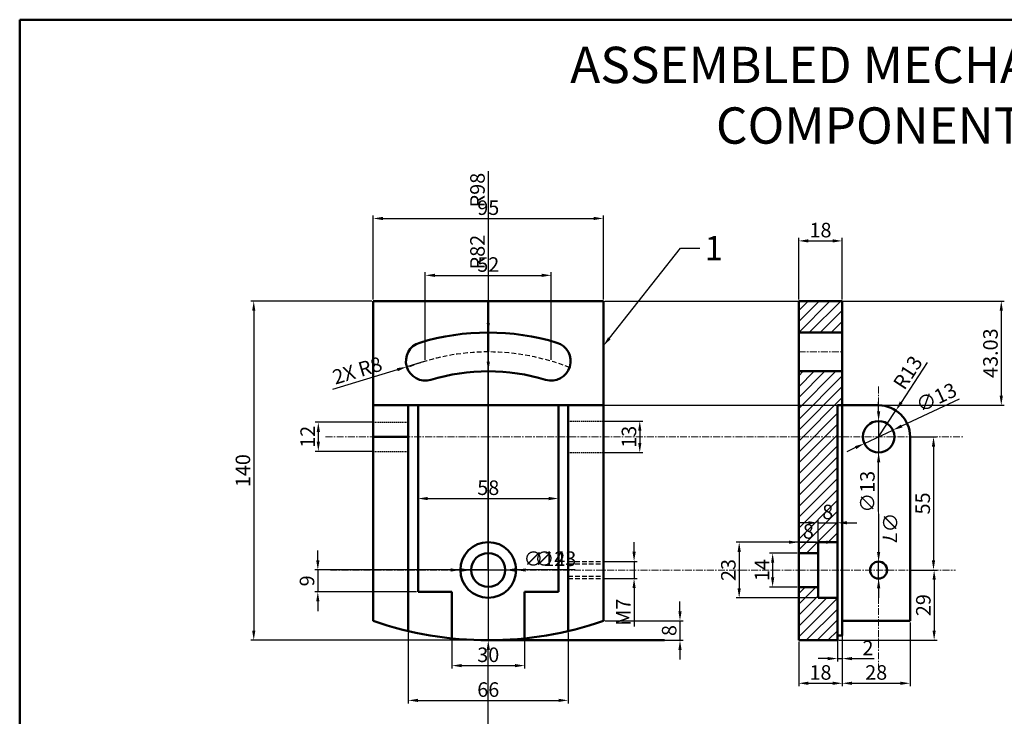
# Model space of a CAD drawing. Units: millimetres. Extents: x 197 to 841, y -182 to 351.
# Tile 2 of 3: x 197 to 603, y 63 to 351. Entities that reach past the tile are written whole.
import ezdxf
from ezdxf import colors
from ezdxf.entities.mleader import LeaderData, LeaderLine
from ezdxf.math import Vec2, Vec3

# ---------------------------------------------------------------- set-up
doc = ezdxf.new("R2010")
doc.units = ezdxf.units.MM
doc.header["$LTSCALE"] = 0.3
doc.linetypes.add('CENTER', pattern=[50.8, 31.75, -6.35, 6.35, -6.35])
doc.linetypes.add('HIDDEN', pattern=[9.525, 6.35, -3.175])
for name, color, linetype, lineweight in [('M-CNTR', 1, 'CENTER', 18), ('M-DIMS', 2, 'Continuous', 25), ('M-HATC', 8, 'Continuous', 18), ('M-HIDN', 6, 'HIDDEN', 25), ('M-OUTL', 7, 'Continuous', 50), ('M-TEXT', 3, 'Continuous', 25), ('M-TTLB', 7, 'Continuous', 50)]:
    doc.layers.add(name, color=color, linetype=linetype, lineweight=lineweight)
doc.styles.get("Standard").update_dxf_attribs({"font": 'arial.ttf'})
doc.dimstyles.new('ISO-25', dxfattribs={"dimtxt": 6, "dimasz": 4, "dimexe": 1.25, "dimexo": 0.625, "dimtad": 1, "dimdec": 0, "dimtxsty": 'Standard', "dimcen": 2.5, "dimadec": 0, "dimazin": 0, "dimtfac": 1, "dimtdec": 0, "dimtmove": 0, "dimatfit": 3, "dimfxl": 1, "dimarcsym": 0})

# ---------------------------------------------------------------- blocks, each defined once
blk = doc.blocks.new('*D1')
at = {"layer": 'Defpoints', "color": 0, "ltscale": 0.3, "transparency": 16777216}
for p in [(536.06, 98.08), (518.06, 94.62), (536.06, 76.86)]:
    blk.add_point(p, dxfattribs=at)
at = {"layer": 'M-DIMS', "color": 0, "lineweight": -2, "ltscale": 0.3, "transparency": 16777216}
for p, q in [((518.06, 94), (518.06, 75.61)), ((536.06, 97.46), (536.06, 75.61)), ((522.06, 76.86), (532.06, 76.86))]:
    blk.add_line(p, q, dxfattribs=at)
at = {"layer": 'M-DIMS', "color": 0, "ltscale": 0.3, "transparency": 16777216}
for points in [[(522.06, 77.52), (522.06, 76.19), (518.06, 76.86)], [(532.06, 77.52), (532.06, 76.19), (536.06, 76.86)]]:
    blk.add_solid(points, dxfattribs=at)
at = {"layer": 'M-DIMS', "color": 0, "ltscale": 0.3, "transparency": 16777216, "insert": (527.06, 80.55), "char_height": 6, "attachment_point": 5}
blk.add_mtext('18', dxfattribs=at)
blk = doc.blocks.new('*D2')
at = {"layer": 'Defpoints', "color": 0, "ltscale": 0.3, "transparency": 16777216}
for p in [(415.93, 245.24), (363.93, 209.78), (415.93, 209.78)]:
    blk.add_point(p, dxfattribs=at)
at = {"layer": 'M-DIMS', "color": 0, "lineweight": -2, "ltscale": 0.3, "transparency": 16777216}
for p, q in [((363.93, 210.41), (363.93, 246.49)), ((367.93, 245.24), (411.93, 245.24)), ((415.93, 210.41), (415.93, 246.49))]:
    blk.add_line(p, q, dxfattribs=at)
at = {"layer": 'M-DIMS', "color": 0, "ltscale": 0.3, "transparency": 16777216}
for points in [[(367.93, 245.91), (367.93, 244.58), (363.93, 245.24)], [(411.93, 245.91), (411.93, 244.58), (415.93, 245.24)]]:
    blk.add_solid(points, dxfattribs=at)
at = {"layer": 'M-DIMS', "color": 0, "ltscale": 0.3, "transparency": 16777216, "insert": (389.93, 248.93), "char_height": 6, "attachment_point": 5}
blk.add_mtext('52', dxfattribs=at)
blk = doc.blocks.new('*D3')
at = {"layer": 'Defpoints', "color": 0, "ltscale": 0.3, "transparency": 16777216}
for p in [(437.43, 268.71), (342.43, 234.62), (437.43, 234.62)]:
    blk.add_point(p, dxfattribs=at)
at = {"layer": 'M-DIMS', "color": 0, "lineweight": -2, "ltscale": 0.3, "transparency": 16777216}
for p, q in [((342.43, 235.25), (342.43, 269.96)), ((346.43, 268.71), (433.43, 268.71)), ((437.43, 235.25), (437.43, 269.96))]:
    blk.add_line(p, q, dxfattribs=at)
at = {"layer": 'M-DIMS', "color": 0, "ltscale": 0.3, "transparency": 16777216}
for points in [[(346.43, 269.38), (346.43, 268.05), (342.43, 268.71)], [(433.43, 269.38), (433.43, 268.05), (437.43, 268.71)]]:
    blk.add_solid(points, dxfattribs=at)
at = {"layer": 'M-DIMS', "color": 0, "ltscale": 0.3, "transparency": 16777216, "insert": (389.93, 272.4), "char_height": 6, "attachment_point": 5}
blk.add_mtext('95', dxfattribs=at)
blk = doc.blocks.new('*D4')
at = {"layer": 'Defpoints', "color": 0, "ltscale": 0.3, "transparency": 16777216}
for p in [(342.43, 234.62), (293.12, 94.62), (389.93, 94.62)]:
    blk.add_point(p, dxfattribs=at)
at = {"layer": 'M-DIMS', "color": 0, "lineweight": -2, "ltscale": 0.3, "transparency": 16777216}
for p, q in [((341.81, 234.62), (291.87, 234.62)), ((293.12, 230.62), (293.12, 98.62)), ((389.31, 94.62), (291.87, 94.62))]:
    blk.add_line(p, q, dxfattribs=at)
at = {"layer": 'M-DIMS', "color": 0, "ltscale": 0.3, "transparency": 16777216}
for points in [[(292.46, 230.62), (293.79, 230.62), (293.12, 234.62)], [(292.46, 98.62), (293.79, 98.62), (293.12, 94.62)]]:
    blk.add_solid(points, dxfattribs=at)
at = {"layer": 'M-DIMS', "color": 0, "ltscale": 0.3, "transparency": 16777216, "insert": (289.43, 164.62), "char_height": 6, "attachment_point": 5, "rotation": 90}
blk.add_mtext('140', dxfattribs=at)
blk = doc.blocks.new('*D5')
at = {"layer": 'Defpoints', "color": 0, "ltscale": 0.3, "transparency": 16777216}
for p in [(389.93, 123.62), (319.57, 114.62), (360.93, 114.62)]:
    blk.add_point(p, dxfattribs=at)
at = {"layer": 'M-DIMS', "color": 0, "lineweight": -2, "ltscale": 0.3, "transparency": 16777216}
for p, q in [((319.57, 127.62), (319.57, 131.62)), ((389.31, 123.62), (318.32, 123.62)), ((319.57, 123.62), (319.57, 114.62)), ((360.31, 114.62), (318.32, 114.62)), ((319.57, 110.62), (319.57, 106.62))]:
    blk.add_line(p, q, dxfattribs=at)
at = {"layer": 'M-DIMS', "color": 0, "ltscale": 0.3, "transparency": 16777216}
for points in [[(318.91, 127.62), (320.24, 127.62), (319.57, 123.62)], [(318.91, 110.62), (320.24, 110.62), (319.57, 114.62)]]:
    blk.add_solid(points, dxfattribs=at)
at = {"layer": 'M-DIMS', "color": 0, "ltscale": 0.3, "transparency": 16777216, "insert": (315.88, 119.12), "char_height": 6, "attachment_point": 5, "rotation": 90}
blk.add_mtext('9', dxfattribs=at)
blk = doc.blocks.new('*D6')
at = {"layer": 'Defpoints', "color": 0, "ltscale": 0.3, "transparency": 16777216}
for p in [(342.43, 184.59), (319.78, 172.59), (342.43, 172.59)]:
    blk.add_point(p, dxfattribs=at)
at = {"layer": 'M-DIMS', "color": 0, "lineweight": -2, "ltscale": 0.3, "transparency": 16777216}
for p, q in [((341.81, 184.59), (318.53, 184.59)), ((319.78, 180.59), (319.78, 176.59)), ((341.81, 172.59), (318.53, 172.59))]:
    blk.add_line(p, q, dxfattribs=at)
at = {"layer": 'M-DIMS', "color": 0, "ltscale": 0.3, "transparency": 16777216}
for points in [[(319.12, 180.59), (320.45, 180.59), (319.78, 184.59)], [(319.12, 176.59), (320.45, 176.59), (319.78, 172.59)]]:
    blk.add_solid(points, dxfattribs=at)
at = {"layer": 'M-DIMS', "color": 0, "ltscale": 0.3, "transparency": 16777216, "insert": (316.15, 178.59), "char_height": 6, "attachment_point": 5, "rotation": 90}
blk.add_mtext('12', dxfattribs=at)
blk = doc.blocks.new('*D7')
at = {"layer": 'Defpoints', "color": 0, "ltscale": 0.3, "transparency": 16777216}
for p in [(437.43, 185.09), (437.43, 172.09), (452.47, 172.09)]:
    blk.add_point(p, dxfattribs=at)
at = {"layer": 'M-DIMS', "color": 0, "lineweight": -2, "ltscale": 0.3, "transparency": 16777216}
for p, q in [((438.06, 185.09), (453.72, 185.09)), ((452.47, 181.09), (452.47, 176.09)), ((438.06, 172.09), (453.72, 172.09))]:
    blk.add_line(p, q, dxfattribs=at)
at = {"layer": 'M-DIMS', "color": 0, "ltscale": 0.3, "transparency": 16777216}
for points in [[(451.81, 181.09), (453.14, 181.09), (452.47, 185.09)], [(451.81, 176.09), (453.14, 176.09), (452.47, 172.09)]]:
    blk.add_solid(points, dxfattribs=at)
at = {"layer": 'M-DIMS', "color": 0, "ltscale": 0.3, "transparency": 16777216, "insert": (448.78, 178.59), "char_height": 6, "attachment_point": 5, "rotation": 90}
blk.add_mtext('13', dxfattribs=at)
blk = doc.blocks.new('*D8')
at = {"layer": 'Defpoints', "color": 0, "ltscale": 0.3, "transparency": 16777216}
for p in [(437.43, 127.12), (437.43, 120.12), (450.13, 120.12)]:
    blk.add_point(p, dxfattribs=at)
at = {"layer": 'M-DIMS', "color": 0, "lineweight": -2, "ltscale": 0.3, "transparency": 16777216}
for p, q in [((450.13, 131.12), (450.13, 135.12)), ((438.06, 127.12), (451.38, 127.12)), ((450.13, 127.12), (450.13, 120.12)), ((438.06, 120.12), (451.38, 120.12)), ((450.13, 116.12), (450.13, 100.23))]:
    blk.add_line(p, q, dxfattribs=at)
at = {"layer": 'M-DIMS', "color": 0, "ltscale": 0.3, "transparency": 16777216}
for points in [[(449.46, 131.12), (450.79, 131.12), (450.13, 127.12)], [(449.46, 116.12), (450.79, 116.12), (450.13, 120.12)]]:
    blk.add_solid(points, dxfattribs=at)
at = {"layer": 'M-DIMS', "color": 0, "ltscale": 0.3, "transparency": 16777216, "insert": (446.5, 106.18), "char_height": 6, "attachment_point": 5, "rotation": 90}
blk.add_mtext('M7', dxfattribs=at)
blk = doc.blocks.new('*D9')
at = {"layer": 'Defpoints', "color": 0, "ltscale": 0.3, "transparency": 16777216}
for p in [(360.93, 153.11), (418.93, 153.11), (418.93, 153.11)]:
    blk.add_point(p, dxfattribs=at)
at = {"layer": 'M-DIMS', "color": 0, "lineweight": -2, "ltscale": 0.3, "transparency": 16777216}
for p, q in [((360.93, 153.73), (360.93, 154.36)), ((364.93, 153.11), (414.93, 153.11)), ((418.93, 153.73), (418.93, 154.36))]:
    blk.add_line(p, q, dxfattribs=at)
at = {"layer": 'M-DIMS', "color": 0, "ltscale": 0.3, "transparency": 16777216}
for points in [[(364.93, 153.77), (364.93, 152.44), (360.93, 153.11)], [(414.93, 153.77), (414.93, 152.44), (418.93, 153.11)]]:
    blk.add_solid(points, dxfattribs=at)
at = {"layer": 'M-DIMS', "color": 0, "ltscale": 0.3, "transparency": 16777216, "insert": (389.93, 156.8), "char_height": 6, "attachment_point": 5}
blk.add_mtext('58', dxfattribs=at)
blk = doc.blocks.new('*D10')
at = {"layer": 'Defpoints', "color": 0, "ltscale": 0.3, "transparency": 16777216}
for p in [(374.93, 95.4), (404.93, 95.4), (404.93, 84.15)]:
    blk.add_point(p, dxfattribs=at)
at = {"layer": 'M-DIMS', "color": 0, "lineweight": -2, "ltscale": 0.3, "transparency": 16777216}
for p, q in [((374.93, 94.77), (374.93, 82.9)), ((404.93, 94.77), (404.93, 82.9)), ((378.93, 84.15), (400.93, 84.15))]:
    blk.add_line(p, q, dxfattribs=at)
at = {"layer": 'M-DIMS', "color": 0, "ltscale": 0.3, "transparency": 16777216}
for points in [[(378.93, 84.82), (378.93, 83.49), (374.93, 84.15)], [(400.93, 84.82), (400.93, 83.49), (404.93, 84.15)]]:
    blk.add_solid(points, dxfattribs=at)
at = {"layer": 'M-DIMS', "color": 0, "ltscale": 0.3, "transparency": 16777216, "insert": (389.93, 87.84), "char_height": 6, "attachment_point": 5}
blk.add_mtext('30', dxfattribs=at)
blk = doc.blocks.new('*D11')
at = {"layer": 'Defpoints', "color": 0, "ltscale": 0.3, "transparency": 16777216}
for p in [(356.93, 98.43), (422.93, 98.43), (422.93, 69.81)]:
    blk.add_point(p, dxfattribs=at)
at = {"layer": 'M-DIMS', "color": 0, "lineweight": -2, "ltscale": 0.3, "transparency": 16777216}
for p, q in [((356.93, 97.8), (356.93, 68.56)), ((422.93, 97.8), (422.93, 68.56)), ((360.93, 69.81), (418.93, 69.81))]:
    blk.add_line(p, q, dxfattribs=at)
at = {"layer": 'M-DIMS', "color": 0, "ltscale": 0.3, "transparency": 16777216}
for points in [[(360.93, 70.47), (360.93, 69.14), (356.93, 69.81)], [(418.93, 70.47), (418.93, 69.14), (422.93, 69.81)]]:
    blk.add_solid(points, dxfattribs=at)
at = {"layer": 'M-DIMS', "color": 0, "ltscale": 0.3, "transparency": 16777216, "insert": (389.93, 73.49), "char_height": 6, "attachment_point": 5}
blk.add_mtext('66', dxfattribs=at)
blk = doc.blocks.new('*D12')
at = {"layer": 'Defpoints', "color": 0, "ltscale": 0.3, "transparency": 16777216}
for p in [(437.43, 102.62), (437.43, 94.62), (469.07, 94.62)]:
    blk.add_point(p, dxfattribs=at)
at = {"layer": 'M-DIMS', "color": 0, "lineweight": -2, "ltscale": 0.3, "transparency": 16777216}
for p, q in [((469.07, 106.62), (469.07, 110.62)), ((438.06, 102.62), (470.32, 102.62)), ((469.07, 102.62), (469.07, 94.62)), ((438.06, 94.62), (470.32, 94.62)), ((469.07, 90.62), (469.07, 86.62))]:
    blk.add_line(p, q, dxfattribs=at)
at = {"layer": 'M-DIMS', "color": 0, "ltscale": 0.3, "transparency": 16777216}
for points in [[(468.41, 106.62), (469.74, 106.62), (469.07, 102.62)], [(468.41, 90.62), (469.74, 90.62), (469.07, 94.62)]]:
    blk.add_solid(points, dxfattribs=at)
at = {"layer": 'M-DIMS', "color": 0, "ltscale": 0.3, "transparency": 16777216, "insert": (465.38, 98.62), "char_height": 6, "attachment_point": 5, "rotation": 90}
blk.add_mtext('8', dxfattribs=at)
blk = doc.blocks.new('*D13')
at = {"layer": 'Defpoints', "color": 0, "ltscale": 0.3, "transparency": 16777216}
for p in [(536.06, 259.45), (518.06, 234.62), (536.06, 234.62)]:
    blk.add_point(p, dxfattribs=at)
at = {"layer": 'M-DIMS', "color": 0, "lineweight": -2, "ltscale": 0.3, "transparency": 16777216}
for p, q in [((518.06, 235.25), (518.06, 260.7)), ((536.06, 235.25), (536.06, 260.7)), ((522.06, 259.45), (532.06, 259.45))]:
    blk.add_line(p, q, dxfattribs=at)
at = {"layer": 'M-DIMS', "color": 0, "ltscale": 0.3, "transparency": 16777216}
for points in [[(522.06, 260.12), (522.06, 258.79), (518.06, 259.45)], [(532.06, 260.12), (532.06, 258.79), (536.06, 259.45)]]:
    blk.add_solid(points, dxfattribs=at)
at = {"layer": 'M-DIMS', "color": 0, "ltscale": 0.3, "transparency": 16777216, "insert": (527.06, 263.14), "char_height": 6, "attachment_point": 5}
blk.add_mtext('18', dxfattribs=at)
blk = doc.blocks.new('*D14')
at = {"layer": 'Defpoints', "color": 0, "ltscale": 0.3, "transparency": 16777216}
for p in [(564.06, 123.59), (534.06, 94.62), (573.98, 94.62)]:
    blk.add_point(p, dxfattribs=at)
at = {"layer": 'M-DIMS', "color": 0, "lineweight": -2, "ltscale": 0.3, "transparency": 16777216}
for p, q in [((564.69, 123.59), (575.23, 123.59)), ((573.98, 119.59), (573.98, 98.62)), ((534.69, 94.62), (575.23, 94.62))]:
    blk.add_line(p, q, dxfattribs=at)
at = {"layer": 'M-DIMS', "color": 0, "ltscale": 0.3, "transparency": 16777216}
for points in [[(573.32, 119.59), (574.65, 119.59), (573.98, 123.59)], [(573.32, 98.62), (574.65, 98.62), (573.98, 94.62)]]:
    blk.add_solid(points, dxfattribs=at)
at = {"layer": 'M-DIMS', "color": 0, "ltscale": 0.3, "transparency": 16777216, "insert": (570.3, 109.11), "char_height": 6, "attachment_point": 5, "rotation": 90}
blk.add_mtext('29', dxfattribs=at)
blk = doc.blocks.new('*D15')
at = {"layer": 'Defpoints', "color": 0, "ltscale": 0.3, "transparency": 16777216}
for p in [(564.06, 178.59), (564.06, 123.59), (573.72, 123.59)]:
    blk.add_point(p, dxfattribs=at)
at = {"layer": 'M-DIMS', "color": 0, "lineweight": -2, "ltscale": 0.3, "transparency": 16777216}
for p, q in [((564.69, 178.59), (574.97, 178.59)), ((573.72, 174.59), (573.72, 127.59)), ((564.69, 123.59), (574.97, 123.59))]:
    blk.add_line(p, q, dxfattribs=at)
at = {"layer": 'M-DIMS', "color": 0, "ltscale": 0.3, "transparency": 16777216}
for points in [[(573.05, 174.59), (574.38, 174.59), (573.72, 178.59)], [(573.05, 127.59), (574.38, 127.59), (573.72, 123.59)]]:
    blk.add_solid(points, dxfattribs=at)
at = {"layer": 'M-DIMS', "color": 0, "ltscale": 0.3, "transparency": 16777216, "insert": (570.04, 151.09), "char_height": 6, "attachment_point": 5, "rotation": 90}
blk.add_mtext('55', dxfattribs=at)
blk = doc.blocks.new('*D16')
at = {"layer": 'Defpoints', "color": 0, "ltscale": 0.3, "transparency": 16777216}
for p in [(518.06, 130.59), (507.31, 116.59), (518.06, 116.59)]:
    blk.add_point(p, dxfattribs=at)
at = {"layer": 'M-DIMS', "color": 0, "lineweight": -2, "ltscale": 0.3, "transparency": 16777216}
for p, q in [((517.44, 130.59), (506.06, 130.59)), ((507.31, 126.59), (507.31, 120.59)), ((517.44, 116.59), (506.06, 116.59))]:
    blk.add_line(p, q, dxfattribs=at)
at = {"layer": 'M-DIMS', "color": 0, "ltscale": 0.3, "transparency": 16777216}
for points in [[(506.64, 126.59), (507.98, 126.59), (507.31, 130.59)], [(506.64, 120.59), (507.98, 120.59), (507.31, 116.59)]]:
    blk.add_solid(points, dxfattribs=at)
at = {"layer": 'M-DIMS', "color": 0, "ltscale": 0.3, "transparency": 16777216, "insert": (503.67, 123.59), "char_height": 6, "attachment_point": 5, "rotation": 90}
blk.add_mtext('14', dxfattribs=at)
blk = doc.blocks.new('*D17')
at = {"layer": 'Defpoints', "color": 0, "ltscale": 0.3, "transparency": 16777216}
for p in [(526.06, 135.09), (493.5, 112.09), (526.06, 112.09)]:
    blk.add_point(p, dxfattribs=at)
at = {"layer": 'M-DIMS', "color": 0, "lineweight": -2, "ltscale": 0.3, "transparency": 16777216}
for p, q in [((525.44, 135.09), (492.25, 135.09)), ((493.5, 131.09), (493.5, 116.09)), ((525.44, 112.09), (492.25, 112.09))]:
    blk.add_line(p, q, dxfattribs=at)
at = {"layer": 'M-DIMS', "color": 0, "ltscale": 0.3, "transparency": 16777216}
for points in [[(492.83, 131.09), (494.17, 131.09), (493.5, 135.09)], [(492.83, 116.09), (494.17, 116.09), (493.5, 112.09)]]:
    blk.add_solid(points, dxfattribs=at)
at = {"layer": 'M-DIMS', "color": 0, "ltscale": 0.3, "transparency": 16777216, "insert": (489.81, 123.59), "char_height": 6, "attachment_point": 5, "rotation": 90}
blk.add_mtext('23', dxfattribs=at)
blk = doc.blocks.new('*D18')
at = {"layer": 'Defpoints', "color": 0, "ltscale": 0.3, "transparency": 16777216}
for p in [(564.06, 102.62), (536.06, 96.62), (564.06, 76.86)]:
    blk.add_point(p, dxfattribs=at)
at = {"layer": 'M-DIMS', "color": 0, "lineweight": -2, "ltscale": 0.3, "transparency": 16777216}
for p, q in [((564.06, 102), (564.06, 75.61)), ((536.06, 96), (536.06, 75.61)), ((540.06, 76.86), (560.06, 76.86))]:
    blk.add_line(p, q, dxfattribs=at)
at = {"layer": 'M-DIMS', "color": 0, "ltscale": 0.3, "transparency": 16777216}
for points in [[(540.06, 77.52), (540.06, 76.19), (536.06, 76.86)], [(560.06, 77.52), (560.06, 76.19), (564.06, 76.86)]]:
    blk.add_solid(points, dxfattribs=at)
at = {"layer": 'M-DIMS', "color": 0, "ltscale": 0.3, "transparency": 16777216, "insert": (550.06, 80.55), "char_height": 6, "attachment_point": 5}
blk.add_mtext('28', dxfattribs=at)
blk = doc.blocks.new('*D19')
at = {"layer": 'Defpoints', "color": 0, "ltscale": 0.3, "transparency": 16777216}
for p in [(534.06, 96.62), (536.06, 96.62), (536.06, 87.05)]:
    blk.add_point(p, dxfattribs=at)
at = {"layer": 'M-DIMS', "color": 0, "lineweight": -2, "ltscale": 0.3, "transparency": 16777216}
for p, q in [((534.06, 96), (534.06, 85.8)), ((536.06, 96), (536.06, 85.8)), ((530.06, 87.05), (526.06, 87.05)), ((534.06, 87.05), (536.06, 87.05)), ((540.06, 87.05), (549.28, 87.05))]:
    blk.add_line(p, q, dxfattribs=at)
at = {"layer": 'M-DIMS', "color": 0, "ltscale": 0.3, "transparency": 16777216}
for points in [[(530.06, 87.71), (530.06, 86.38), (534.06, 87.05)], [(540.06, 87.71), (540.06, 86.38), (536.06, 87.05)]]:
    blk.add_solid(points, dxfattribs=at)
at = {"layer": 'M-DIMS', "color": 0, "ltscale": 0.3, "transparency": 16777216, "insert": (546.67, 90.68), "char_height": 6, "attachment_point": 5}
blk.add_mtext('2', dxfattribs=at)
blk = doc.blocks.new('*D20')
at = {"layer": 'Defpoints', "color": 0, "ltscale": 0.3, "transparency": 16777216}
for p in [(534.06, 143.11), (526.06, 135.09), (534.06, 135.09)]:
    blk.add_point(p, dxfattribs=at)
at = {"layer": 'M-DIMS', "color": 0, "lineweight": -2, "ltscale": 0.3, "transparency": 16777216}
for p, q in [((522.06, 143.11), (518.06, 143.11)), ((526.06, 135.72), (526.06, 144.36)), ((526.06, 143.11), (534.06, 143.11)), ((534.06, 135.72), (534.06, 144.36)), ((538.06, 143.11), (542.06, 143.11))]:
    blk.add_line(p, q, dxfattribs=at)
at = {"layer": 'M-DIMS', "color": 0, "ltscale": 0.3, "transparency": 16777216}
for points in [[(522.06, 143.77), (522.06, 142.44), (526.06, 143.11)], [(538.06, 143.77), (538.06, 142.44), (534.06, 143.11)]]:
    blk.add_solid(points, dxfattribs=at)
at = {"layer": 'M-DIMS', "color": 0, "ltscale": 0.3, "transparency": 16777216, "insert": (530.06, 146.8), "char_height": 6, "attachment_point": 5}
blk.add_mtext('8', dxfattribs=at)
blk = doc.blocks.new('*D21')
at = {"layer": 'Defpoints', "color": 0, "ltscale": 0.3, "transparency": 16777216}
for p in [(526.06, 135.09), (518.06, 130.59), (526.06, 130.59)]:
    blk.add_point(p, dxfattribs=at)
at = {"layer": 'M-DIMS', "color": 0, "lineweight": -2, "ltscale": 0.3, "transparency": 16777216}
for p, q in [((514.06, 135.09), (510.06, 135.09)), ((518.06, 131.22), (518.06, 136.34)), ((518.06, 135.09), (526.06, 135.09)), ((526.06, 131.22), (526.06, 136.34)), ((530.06, 135.09), (534.06, 135.09))]:
    blk.add_line(p, q, dxfattribs=at)
at = {"layer": 'M-DIMS', "color": 0, "ltscale": 0.3, "transparency": 16777216}
for points in [[(514.06, 135.76), (514.06, 134.43), (518.06, 135.09)], [(530.06, 135.76), (530.06, 134.43), (526.06, 135.09)]]:
    blk.add_solid(points, dxfattribs=at)
at = {"layer": 'M-DIMS', "color": 0, "ltscale": 0.3, "transparency": 16777216, "insert": (522.06, 138.78), "char_height": 6, "attachment_point": 5}
blk.add_mtext('8', dxfattribs=at)
blk = doc.blocks.new('*D22')
at = {"layer": 'Defpoints', "color": 0, "ltscale": 0.3, "transparency": 16777216}
for p in [(558.18, 189.47), (551.06, 178.59)]:
    blk.add_point(p, dxfattribs=at)
at = {"layer": 'M-DIMS', "color": 0, "lineweight": -2, "ltscale": 0.3, "transparency": 16777216}
for p, q in [((571.11, 209.2), (560.38, 192.81)), ((551.06, 178.59), (558.18, 189.47))]:
    blk.add_line(p, q, dxfattribs=at)
at = {"layer": 'M-DIMS', "color": 0, "ltscale": 0.3, "transparency": 16777216}
blk.add_solid([(559.82, 193.18), (560.93, 192.45), (558.18, 189.47)], dxfattribs=at)
at = {"layer": 'M-DIMS', "color": 0, "ltscale": 0.3, "transparency": 16777216, "insert": (563.75, 204.7), "char_height": 6, "attachment_point": 5, "rotation": 56.7737}
blk.add_mtext('R13', dxfattribs=at)
blk = doc.blocks.new('*D23')
at = {"layer": 'Defpoints', "color": 0, "ltscale": 0.3, "transparency": 16777216}
for p in [(556.95, 181.35), (545.17, 175.84)]:
    blk.add_point(p, dxfattribs=at)
at = {"layer": 'M-DIMS', "color": 0, "lineweight": -2, "ltscale": 0.3, "transparency": 16777216}
for p, q in [((584.27, 194.14), (560.57, 183.05)), ((545.17, 175.84), (556.95, 181.35)), ((541.55, 174.14), (537.93, 172.44))]:
    blk.add_line(p, q, dxfattribs=at)
at = {"layer": 'M-DIMS', "color": 0, "ltscale": 0.3, "transparency": 16777216}
for points in [[(560.29, 183.65), (560.85, 182.44), (556.95, 181.35)], [(541.27, 174.74), (541.83, 173.54), (545.17, 175.84)]]:
    blk.add_solid(points, dxfattribs=at)
at = {"layer": 'M-DIMS', "color": 0, "ltscale": 0.3, "transparency": 16777216, "insert": (575.22, 194.16), "char_height": 6, "attachment_point": 5, "rotation": 25.0912}
blk.add_mtext('∅13', dxfattribs=at)
blk = doc.blocks.new('*D64')
at = {"layer": 'Defpoints', "color": 0, "ltscale": 0.3, "transparency": 16777216}
for p in [(437.43, 234.62), (437.43, 191.59), (601.69, 191.59)]:
    blk.add_point(p, dxfattribs=at)
at = {"layer": 'M-DIMS', "color": 0, "lineweight": -2, "ltscale": 0.3, "transparency": 16777216}
for p, q in [((438.06, 234.62), (602.94, 234.62)), ((601.69, 230.62), (601.69, 195.59)), ((438.06, 191.59), (602.94, 191.59))]:
    blk.add_line(p, q, dxfattribs=at)
at = {"layer": 'M-DIMS', "color": 0, "ltscale": 0.3, "transparency": 16777216}
for points in [[(601.02, 230.62), (602.36, 230.62), (601.69, 234.62)], [(601.02, 195.59), (602.36, 195.59), (601.69, 191.59)]]:
    blk.add_solid(points, dxfattribs=at)
at = {"layer": 'M-DIMS', "color": 0, "ltscale": 0.3, "transparency": 16777216, "insert": (598, 213.11), "char_height": 6, "attachment_point": 5, "rotation": 90}
blk.add_mtext('43.03', dxfattribs=at)
blk = doc.blocks.new('*D67')
at = {"layer": 'Defpoints', "color": 0, "ltscale": 0.3, "transparency": 16777216}
for p in [(356.28, 207.47), (363.93, 209.78)]:
    blk.add_point(p, dxfattribs=at)
at = {"layer": 'M-DIMS', "color": 0, "lineweight": -2, "ltscale": 0.3, "transparency": 16777216}
for p, q in [((363.93, 209.78), (356.28, 207.47)), ((325.71, 198.25), (352.45, 206.32))]:
    blk.add_line(p, q, dxfattribs=at)
at = {"layer": 'M-DIMS', "color": 0, "ltscale": 0.3, "transparency": 16777216}
blk.add_solid([(352.25, 206.95), (352.64, 205.68), (356.28, 207.47)], dxfattribs=at)
at = {"layer": 'M-DIMS', "color": 0, "ltscale": 0.3, "transparency": 16777216, "insert": (336.1, 205.23), "char_height": 6, "attachment_point": 5, "rotation": 16.7934}
blk.add_mtext('2X R8', dxfattribs=at)
blk = doc.blocks.new('*D68')
at = {"layer": 'Defpoints', "color": 0, "ltscale": 0.3, "transparency": 16777216}
for p in [(389.94, 221.62), (389.93, 123.62)]:
    blk.add_point(p, dxfattribs=at)
at = {"layer": 'M-DIMS', "color": 0, "lineweight": -2, "ltscale": 0.3, "transparency": 16777216}
for p, q in [((389.94, 288.22), (389.94, 225.62)), ((389.93, 123.62), (389.94, 221.62))]:
    blk.add_line(p, q, dxfattribs=at)
at = {"layer": 'M-DIMS', "color": 0, "ltscale": 0.3, "transparency": 16777216}
blk.add_solid([(389.27, 225.62), (390.6, 225.62), (389.94, 221.62)], dxfattribs=at)
at = {"layer": 'M-DIMS', "color": 0, "ltscale": 0.3, "transparency": 16777216, "insert": (386.25, 280.42), "char_height": 6, "attachment_point": 5, "rotation": 89.9999}
blk.add_mtext('R98', dxfattribs=at)
blk = doc.blocks.new('*D69')
at = {"layer": 'Defpoints', "color": 0, "ltscale": 0.3, "transparency": 16777216}
for p in [(389.93, 205.62), (389.93, 123.62)]:
    blk.add_point(p, dxfattribs=at)
at = {"layer": 'M-DIMS', "color": 0, "lineweight": -2, "ltscale": 0.3, "transparency": 16777216}
for p, q in [((389.94, 262.58), (389.93, 209.62)), ((389.93, 123.62), (389.93, 205.62))]:
    blk.add_line(p, q, dxfattribs=at)
at = {"layer": 'M-DIMS', "color": 0, "ltscale": 0.3, "transparency": 16777216}
blk.add_solid([(389.27, 209.62), (390.6, 209.62), (389.93, 205.62)], dxfattribs=at)
at = {"layer": 'M-DIMS', "color": 0, "ltscale": 0.3, "transparency": 16777216, "insert": (386.25, 254.82), "char_height": 6, "attachment_point": 5, "rotation": 89.9999}
blk.add_mtext('R82', dxfattribs=at)
blk = doc.blocks.new('*D70')
at = {"layer": 'Defpoints', "color": 0, "ltscale": 0.3, "transparency": 16777216}
for p in [(389.93, 239.64), (389.94, 94.62)]:
    blk.add_point(p, dxfattribs=at)
at = {"layer": 'M-DIMS', "color": 0, "lineweight": -2, "ltscale": 0.3, "transparency": 16777216}
for p, q in [((389.93, 239.64), (389.94, 94.62)), ((389.94, -8.31), (389.94, 90.62))]:
    blk.add_line(p, q, dxfattribs=at)
at = {"layer": 'M-DIMS', "color": 0, "ltscale": 0.3, "transparency": 16777216}
blk.add_solid([(390.6, 90.62), (389.27, 90.62), (389.94, 94.62)], dxfattribs=at)
at = {"layer": 'M-DIMS', "color": 0, "ltscale": 0.3, "transparency": 16777216, "insert": (393.62, 7.61), "char_height": 6, "attachment_point": 5, "rotation": 270.0001}
blk.add_mtext('R145.02', dxfattribs=at)
blk = doc.blocks.new('*D71')
at = {"layer": 'Defpoints', "color": 0, "ltscale": 0.3, "transparency": 16777216}
for p in [(378.43, 123.62), (401.43, 123.62)]:
    blk.add_point(p, dxfattribs=at)
at = {"layer": 'M-DIMS', "color": 0, "lineweight": -2, "ltscale": 0.3, "transparency": 16777216}
for p, q in [((374.43, 123.62), (370.43, 123.62)), ((378.43, 123.62), (401.43, 123.62)), ((425.81, 123.62), (405.43, 123.62))]:
    blk.add_line(p, q, dxfattribs=at)
at = {"layer": 'M-DIMS', "color": 0, "ltscale": 0.3, "transparency": 16777216}
for points in [[(374.43, 124.29), (374.43, 122.95), (378.43, 123.62)], [(405.43, 124.29), (405.43, 122.95), (401.43, 123.62)]]:
    blk.add_solid(points, dxfattribs=at)
at = {"layer": 'M-DIMS', "color": 0, "ltscale": 0.3, "transparency": 16777216, "insert": (417.62, 127.48), "char_height": 6, "attachment_point": 5, "rotation": 0.0013}
blk.add_mtext('∅23', dxfattribs=at)
blk = doc.blocks.new('*D72')
at = {"layer": 'Defpoints', "color": 0, "ltscale": 0.3, "transparency": 16777216}
for p in [(382.93, 123.62), (396.93, 123.62)]:
    blk.add_point(p, dxfattribs=at)
at = {"layer": 'M-DIMS', "color": 0, "lineweight": -2, "ltscale": 0.3, "transparency": 16777216}
for p, q in [((378.93, 123.62), (374.93, 123.62)), ((382.93, 123.62), (396.93, 123.62)), ((421.28, 123.62), (400.93, 123.62))]:
    blk.add_line(p, q, dxfattribs=at)
at = {"layer": 'M-DIMS', "color": 0, "ltscale": 0.3, "transparency": 16777216}
for points in [[(378.93, 124.29), (378.93, 122.95), (382.93, 123.62)], [(400.93, 124.29), (400.93, 122.95), (396.93, 123.62)]]:
    blk.add_solid(points, dxfattribs=at)
at = {"layer": 'M-DIMS', "color": 0, "ltscale": 0.3, "transparency": 16777216, "insert": (413.11, 127.48), "char_height": 6, "attachment_point": 5, "rotation": 0.0022}
blk.add_mtext('∅14', dxfattribs=at)
blk = doc.blocks.new('*D73')
at = {"layer": 'Defpoints', "color": 0, "ltscale": 0.3, "transparency": 16777216}
for p in [(551.06, 185.09), (551.06, 172.09)]:
    blk.add_point(p, dxfattribs=at)
at = {"layer": 'M-DIMS', "color": 0, "lineweight": -2, "ltscale": 0.3, "transparency": 16777216}
for p, q in [((551.06, 189.09), (551.06, 193.09)), ((551.06, 185.09), (551.06, 172.09)), ((551.06, 147.72), (551.06, 168.09))]:
    blk.add_line(p, q, dxfattribs=at)
at = {"layer": 'M-DIMS', "color": 0, "ltscale": 0.3, "transparency": 16777216}
for points in [[(550.39, 189.09), (551.73, 189.09), (551.06, 185.09)], [(550.39, 168.09), (551.73, 168.09), (551.06, 172.09)]]:
    blk.add_solid(points, dxfattribs=at)
at = {"layer": 'M-DIMS', "color": 0, "ltscale": 0.3, "transparency": 16777216, "insert": (547.2, 155.91), "char_height": 6, "attachment_point": 5, "rotation": 89.9987}
blk.add_mtext('∅13', dxfattribs=at)
blk = doc.blocks.new('*D74')
at = {"layer": 'Defpoints', "color": 0, "ltscale": 0.3, "transparency": 16777216}
for p in [(551.06, 127.09), (551.06, 120.09)]:
    blk.add_point(p, dxfattribs=at)
at = {"layer": 'M-DIMS', "color": 0, "lineweight": -2, "ltscale": 0.3, "transparency": 16777216}
for p, q in [((551.06, 146.8), (551.06, 131.09)), ((551.06, 120.09), (551.06, 127.09)), ((551.06, 116.09), (551.06, 112.09))]:
    blk.add_line(p, q, dxfattribs=at)
at = {"layer": 'M-DIMS', "color": 0, "ltscale": 0.3, "transparency": 16777216}
for points in [[(551.73, 131.09), (550.39, 131.09), (551.06, 127.09)], [(551.73, 116.09), (550.39, 116.09), (551.06, 120.09)]]:
    blk.add_solid(points, dxfattribs=at)
at = {"layer": 'M-DIMS', "color": 0, "ltscale": 0.3, "transparency": 16777216, "insert": (554.92, 140.95), "char_height": 6, "attachment_point": 5, "rotation": 270.0025}
blk.add_mtext('∅7', dxfattribs=at)

msp = doc.modelspace()

# ---------------------------------------------------------------- hatches: boundary and pattern name
at = {"layer": 'M-HATC', "ltscale": 0.3}
h = msp.add_hatch(dxfattribs=at)
h.set_pattern_fill('ANSI31', color=256)
h.paths.add_polyline_path([(534.0602, 178.5927), (518.0602, 178.5927), (518.0602, 130.5927), (526.0602, 130.5927), (526.0602, 135.0927), (534.0602, 135.0927)])
h.paths.add_polyline_path([(534.0602, 112.0927), (526.0602, 112.0927), (526.0602, 116.5927), (518.0602, 116.5927), (518.0602, 94.6207), (534.0602, 94.6207)])
h.paths.add_polyline_path([(536.0602, 205.6207), (518.0602, 205.6207), (518.0602, 178.5927), (534.0602, 178.5927), (534.0602, 191.5927), (536.0602, 191.5927)])
h.paths.add_polyline_path([(536.0602, 234.6207), (518.0602, 234.6207), (518.0602, 221.6207), (536.0602, 221.6207)])

# ---------------------------------------------------------------- linework, layer by layer
at = {"layer": 'M-CNTR'}
msp.add_line((389.9348, 234.6207), (389.9348, 94.6207), dxfattribs=at)
at = {"layer": 'M-CNTR', "ltscale": 0.3}
for p, q in [((518.0602, 213.6207), (536.0602, 213.6207)), ((551.0602, 199.3431), (551.0602, 83.5004)), ((322.7995, 178.5927), (536.0602, 178.5927)), ((536.0602, 178.5927), (586.0907, 178.5927)), ((324.7426, 123.5927), (518.0602, 123.5927)), ((518.0602, 123.5927), (582.811, 123.5927))]:
    msp.add_line(p, q, dxfattribs=at)
at = {"layer": 'M-HIDN', "ltscale": 0.3}
for p, q in [((342.4348, 184.5927), (356.9348, 184.5927)), ((422.9348, 185.0927), (437.4348, 185.0927)), ((342.4348, 172.5927), (356.9348, 172.5927)), ((422.9348, 172.0927), (437.4348, 172.0927))]:
    msp.add_line(p, q, dxfattribs=at)
at = {"layer": 'M-HIDN'}
for p, q in [((422.9348, 127.1207), (437.4348, 127.1207)), ((422.9348, 126.1207), (437.4348, 126.1207)), ((422.9348, 121.1207), (437.4348, 121.1207)), ((422.9348, 120.1207), (437.4348, 120.1207))]:
    msp.add_line(p, q, dxfattribs=at)
msp.add_arc((389.9348, 123.6207), 90, 68.113917, 111.886083, dxfattribs=at)
at = {"layer": 'M-OUTL'}
for p, q in [((342.4348, 234.6207), (437.4348, 234.6207)), ((342.4348, 102.6207), (342.4348, 234.6207)), ((389.9348, 234.6207), (389.9348, 213.6207)), ((437.4348, 234.6207), (437.4348, 102.6207)), ((356.9348, 98.4254), (356.9348, 191.5927)), ((360.9348, 191.5927), (360.9348, 114.6207)), ((418.9348, 191.5927), (418.9348, 114.6207)), ((422.9348, 98.4254), (422.9348, 191.5927)), ((360.9348, 114.6207), (374.9348, 114.6207)), ((374.9348, 95.3986), (374.9348, 114.6207)), ((404.9348, 95.3986), (404.9348, 114.6207)), ((404.9348, 114.6207), (418.9348, 114.6207))]:
    msp.add_line(p, q, dxfattribs=at)
at = {"layer": 'M-OUTL', "ltscale": 0.3}
for p, q in [((518.0602, 94.6207), (518.0602, 234.6207)), ((518.0602, 234.6207), (536.0602, 234.6207)), ((536.0602, 234.6207), (536.0602, 96.6207)), ((518.0602, 221.6207), (536.0602, 221.6207)), ((518.0602, 205.6207), (536.0602, 205.6207)), ((437.4348, 191.5927), (342.4348, 191.5927)), ((534.0602, 191.5927), (534.0602, 94.6207)), ((534.0602, 191.5927), (551.0602, 191.5927)), ((342.4348, 178.5927), (356.9348, 178.5927)), ((564.0602, 178.5927), (564.0602, 102.6207)), ((526.0602, 135.0927), (534.0602, 135.0927)), ((526.0602, 112.0927), (526.0602, 135.0927)), ((518.0602, 130.5927), (526.0602, 130.5927)), ((518.0602, 116.5927), (526.0602, 116.5927)), ((526.0602, 112.0927), (534.0602, 112.0927)), ((536.0602, 102.6207), (564.0602, 102.6207)), ((389.9348, 94.6207), (462.6116, 94.6207)), ((534.0602, 94.6207), (518.0602, 94.6207)), ((534.0602, 96.6207), (536.0602, 96.6207))]:
    msp.add_line(p, q, dxfattribs=at)
for centre, radius in [((551.0602, 178.5927), 6.5), ((551.0602, 123.5927), 3.5)]:
    msp.add_circle(centre, radius, dxfattribs=at)
at = {"layer": 'M-OUTL'}
for radius in [11.5, 7]:
    msp.add_circle((389.9348, 123.6207), radius, dxfattribs=at)
for centre, radius, start, end in [((389.9348, 123.6207), 98, 73.208553, 106.791447), ((363.9348, 209.7834), 8, 106.791447, 286.791447), ((415.9348, 209.7834), 8, 253.208553, 73.208553), ((389.9348, 123.6207), 82, 73.208553, 106.791447)]:
    msp.add_arc(centre, radius, start, end, dxfattribs=at)
at = {"layer": 'M-OUTL', "ltscale": 0.3}
for centre, radius, start, end in [((551.0602, 178.5927), 13, 0, 90), ((389.9348, 239.6364), 145.0156, 250.879807, 289.120193)]:
    msp.add_arc(centre, radius, start, end, dxfattribs=at)
at = {"layer": 'M-TTLB', "ltscale": 0.3}
msp.add_lwpolyline([(196.5121, 350.7597), (840.9228, 350.7597), (840.9228, -131.7005), (196.5121, -131.7005)], close=True, dxfattribs=at)

# ---------------------------------------------------------------- texts
at = {"layer": 'M-TEXT', "ltscale": 0.3, "insert": (410.4687, 339.5846), "char_height": 15, "attachment_point": 1}
msp.add_mtext_dynamic_manual_height_columns('\\pxqc;ASSEMBLED MECHANICAL COMPONENT', width=273.781942, gutter_width=12.5, heights=[0], dxfattribs=at)

# ---------------------------------------------------------------- dimensions: what is measured, and where the dimension line sits
at = {"layer": 'M-DIMS', "ltscale": 0.3}
for center, mpoint, override, picture, middle in [((389.9348, 123.6207), (389.935, 221.6207), {"dimdec": 0, "dimlfac": 1, "dimrnd": 0, "dimzin": 0, "dimdsep": 46, "dimlunit": 2}, '*D68', (389.9351, 280.4207)), ((389.9348, 123.6207), (389.935, 205.6207), {"dimdec": 0, "dimlfac": 1, "dimrnd": 0, "dimzin": 0, "dimdsep": 46, "dimlunit": 2}, '*D69', (389.9351, 254.8207)), ((389.9348, 239.6364), (389.935, 94.6207), {"dimdec": 2, "dimlfac": 1, "dimrnd": 0, "dimzin": 0, "dimdsep": 46, "dimlunit": 2}, '*D70', (389.9351, 7.6114))]:
    dim = msp.add_radius_dim(center=center, mpoint=mpoint, dimstyle='ISO-25', override=override, dxfattribs=at)
    dim.commit()
    dim.dimension.update_dxf_attribs({"geometry": picture, "text_midpoint": middle, "dimtype": 164})
for base, p1, p2, picture, middle in [((437.4348, 268.7134), (342.4348, 234.6207), (437.4348, 234.6207), '*D3', (389.9348, 272.4019)), ((536.0602, 259.4518), (518.0602, 234.6207), (536.0602, 234.6207), '*D13', (527.0602, 263.1402)), ((415.9348, 245.2419), (363.9348, 209.7834), (415.9348, 209.7834), '*D2', (389.9348, 248.9304)), ((418.9348, 153.1067), (360.9348, 153.1067), (418.9348, 153.1067), '*D9', (389.9348, 156.7951)), ((534.0602, 143.1067), (526.0602, 135.0927), (534.0602, 135.0927), '*D20', (530.0602, 146.7951)), ((526.0602, 135.0927), (518.0602, 130.5927), (526.0602, 130.5927), '*D21', (522.0602, 138.7811)), ((564.0602, 76.8567), (536.0602, 96.6207), (564.0602, 102.6207), '*D18', (550.0602, 80.5451)), ((422.9348, 69.8055), (356.9348, 98.4254), (422.9348, 98.4254), '*D11', (389.9348, 73.494)), ((536.0602, 76.8567), (518.0602, 94.6207), (536.0602, 98.0848), '*D1', (527.0602, 80.5451)), ((404.9348, 84.1536), (374.9348, 95.3986), (404.9348, 95.3986), '*D10', (389.9348, 87.844)), ((536.0602, 87.0465), (534.0602, 96.6207), (536.0602, 96.6207), '*D19', (546.6722, 90.6838))]:
    dim = msp.add_linear_dim(base=base, p1=p1, p2=p2, dimstyle='ISO-25', override={"dimclrd": 0, "dimclre": 0, "dimclrt": 0}, dxfattribs=at)
    dim.commit()
    dim.dimension.update_dxf_attribs({"geometry": picture, "text_midpoint": middle})
for base, p1, p2, override, picture, middle in [((293.1221, 94.6207), (342.4348, 234.6207), (389.9348, 94.6207), {"dimclrd": 0, "dimclre": 0, "dimclrt": 0}, '*D4', (289.4336, 164.6207)), ((601.6907, 191.5927), (437.4348, 234.6207), (437.4348, 191.5927), {"dimdec": 2, "dimlfac": 1, "dimrnd": 0, "dimzin": 0, "dimdsep": 46, "dimlunit": 2}, '*D64', (598.0002, 213.1067)), ((319.7838, 172.5927), (342.4348, 184.5927), (342.4348, 172.5927), {"dimclrd": 0, "dimclre": 0, "dimclrt": 0}, '*D6', (316.1465, 178.5927)), ((452.4729, 172.0927), (437.4348, 185.0927), (437.4348, 172.0927), {"dimclrd": 0, "dimclre": 0, "dimclrt": 0}, '*D7', (448.7824, 178.5927)), ((573.7155, 123.5927), (564.0602, 178.5927), (564.0602, 123.5927), {"dimclrd": 0, "dimclre": 0, "dimclrt": 0}, '*D15', (570.0393, 151.0927)), ((493.5002, 112.0927), (526.0602, 135.0927), (526.0602, 112.0927), {"dimclrd": 0, "dimclre": 0, "dimclrt": 0}, '*D17', (489.8097, 123.5927)), ((319.5731, 114.6207), (389.9348, 123.6207), (360.9348, 114.6207), {"dimclrd": 0, "dimclre": 0, "dimclrt": 0}, '*D5', (315.8846, 119.1207)), ((507.3093, 116.5927), (518.0602, 130.5927), (518.0602, 116.5927), {"dimclrd": 0, "dimclre": 0, "dimclrt": 0}, '*D16', (503.672, 123.5927)), ((573.9837, 94.6207), (564.0602, 123.5927), (534.0602, 94.6207), {"dimclrd": 0, "dimclre": 0, "dimclrt": 0}, '*D14', (570.2953, 109.1067)), ((469.0724, 94.6207), (437.4348, 102.6207), (437.4348, 94.6207), {"dimclrd": 0, "dimclre": 0, "dimclrt": 0}, '*D12', (465.384, 98.6207))]:
    dim = msp.add_linear_dim(base=base, p1=p1, p2=p2, angle=90, dimstyle='ISO-25', override=override, dxfattribs=at)
    dim.commit()
    dim.dimension.update_dxf_attribs({"geometry": picture, "text_midpoint": middle})
dim = msp.add_radius_dim(center=(363.9348, 209.7834), mpoint=(356.276, 207.472), text='2X <>', dimstyle='ISO-25', override={"dimdec": 0, "dimlfac": 1, "dimrnd": 0, "dimzin": 0, "dimdsep": 46, "dimlunit": 2}, dxfattribs=at)
dim.commit()
dim.dimension.update_dxf_attribs({"geometry": '*D67', "text_midpoint": (336.0958, 205.2345)})
dim = msp.add_radius_dim(center=(551.0602, 178.5927), mpoint=(558.1835, 189.4674), dimstyle='ISO-25', override={"dimclrd": 0, "dimclre": 0, "dimclrt": 0}, dxfattribs=at)
dim.commit()
dim.dimension.update_dxf_attribs({"geometry": '*D22', "text_midpoint": (563.7503, 204.701)})
for p1, p2, override, picture, middle in [((545.1735, 175.8363), (556.9468, 181.3491), {"dimclrd": 0, "dimclre": 0, "dimclrt": 0}, '*D23', (576.855, 190.6711)), ((378.4348, 123.6205), (401.4348, 123.621), {"dimdec": 0, "dimlfac": 1, "dimrnd": 0, "dimzin": 0, "dimdsep": 46, "dimlunit": 2}, '*D71', (417.6212, 123.6214)), ((382.9348, 123.6205), (396.9348, 123.621), {"dimdec": 0, "dimlfac": 1, "dimrnd": 0, "dimzin": 0, "dimdsep": 46, "dimlunit": 2}, '*D72', (413.1089, 123.6216))]:
    dim = msp.add_diameter_dim_2p(p1=p1, p2=p2, dimstyle='ISO-25', override=override, dxfattribs=at)
    dim.commit()
    dim.dimension.update_dxf_attribs({"geometry": picture, "text_midpoint": middle, "dimtype": 163})
for p1, p2, picture, middle in [((551.0603, 185.0927), (551.06, 172.0927), '*D73', (551.0596, 155.9063)), ((551.0603, 120.0927), (551.06, 127.0927), '*D74', (551.0594, 140.9483))]:
    dim = msp.add_diameter_dim_2p(p1=p1, p2=p2, dimstyle='ISO-25', override={"dimdec": 0, "dimlfac": 1, "dimrnd": 0, "dimzin": 0, "dimdsep": 46, "dimlunit": 2}, dxfattribs=at)
    dim.commit()
    dim.dimension.update_dxf_attribs({"geometry": picture, "text_midpoint": middle})
dim = msp.add_linear_dim(base=(450.1266, 120.1207), p1=(437.4348, 127.1207), p2=(437.4348, 120.1207), angle=90, text='M<>', dimstyle='ISO-25', override={"dimclrd": 0, "dimclre": 0, "dimclrt": 0}, dxfattribs=at)
dim.commit()
dim.dimension.update_dxf_attribs({"geometry": '*D8', "text_midpoint": (446.5016, 106.1751)})

# ---------------------------------------------------------------- leaders
ml = msp.add_multileader_mtext('Standard', dxfattribs=at)
ml.set_content('1', color=256)
ml.set_leader_properties()
ml.build(insert=Vec2(0, 0))
ctx = ml.context
ctx.base_point, ctx.char_height, ctx.plane_origin = Vec3(477.2269, 256.4443), 10, Vec3(437.4348, 216.1203)
notes = []
notes.append((ctx, [(0, (1, 1, 0), (469.2269, 256.4443), (1, 0), 8, [(0, [(437.4348, 216.1203)], 0, [])])]))
ctx.mtext.insert, ctx.mtext.flow_direction = Vec3(479.2269, 261.4443), 5
for ctx, leaders in notes:
    for number, flags, end, landing, length, lines in leaders:
        leader = LeaderData()
        leader.index, (leader.has_last_leader_line, leader.has_dogleg_vector, leader.attachment_direction) = number, flags
        leader.last_leader_point, leader.dogleg_vector, leader.dogleg_length = Vec3(end), Vec3(landing), length
        for number, points, colour, breaks in lines:
            line = LeaderLine()
            line.index, line.vertices, line.color, line.breaks = number, Vec3.list(points), colors.encode_raw_color(colour), breaks
            leader.lines.append(line)
        ctx.leaders.append(leader)

doc.saveas('drawing.dxf')
